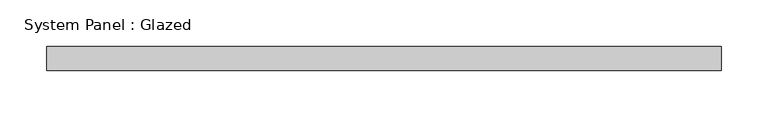
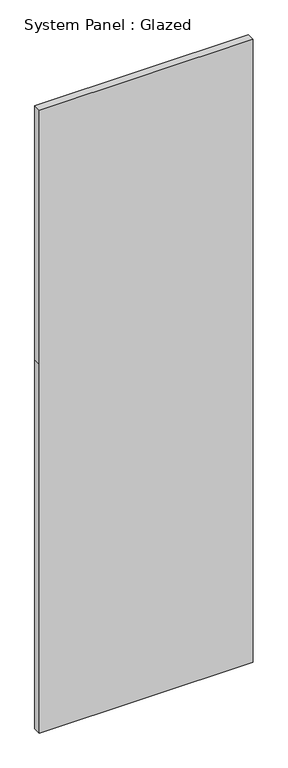
"""IFC4 building model written with IfcOpenShell, lengths in millimetres: plate geometry, System Panel : Glazed."""

from ifc_helpers import new_model, si_unit, frame, origin, place, context, project, spatial, polyline, outline, extrude, source, transform, mapped, element, save


def system_panel_glazed_9a0fbd8e(model_context):
    return source(origin(), model_context, "Body", "SweptSolid", [
        extrude(outline(polyline([(0.0, -358.775), (0.0, 358.775), (1308.1, 358.775), (2209.8, 358.775), (2209.8, -358.775), (1308.1, -358.775), (0.0, -358.775)])), frame((0.0, 19.05, 0.0), z_axis=(0.0, 1.0, 0.0), x_axis=(0.0, 0.0, 1.0)), (0.0, 0.0, 1.0), 25.4),
    ])


if __name__ == "__main__":
    model = new_model("IFC4")
    model_context = context("Model", 3, world=origin())
    ifc_project = project(units=[si_unit("LENGTHUNIT", "METRE", prefix="MILLI")], contexts=[model_context])
    site = spatial("IfcSite", under=ifc_project)
    building = spatial("IfcBuilding", under=site)
    placement = place(None, origin())
    system_panel_glazed_shape = system_panel_glazed_9a0fbd8e(model_context)
    element("IfcPlate", 1, ObjectType="System Panel : Glazed", at=placement, inside=building, context=model_context, shape_type="MappedRepresentation", body=[
        mapped(system_panel_glazed_shape, transform((0.0, 0.0, 0.0), x_axis=(1.0, 0.0, 0.0), y_axis=(0.0, 1.0, 0.0), z_axis=(0.0, 0.0, 1.0))),
    ])
    save(model, "model.ifc")

# Revit data of these elements
# Type "System Panel : Glazed"
#   Construction Type Id = "GSP4R"
#   Analytic Construction = "1/8 in Pilkington single glazing"
#   Visual Light Transmittance = 0.9
#   Solar Heat Gain Coefficient = 0.86
#   Heat Transfer Coefficient (U) = 1.18115 BTU/(h·ft²·°F)
#   Define Thermal Properties by = 1
# Element 1 (IfcPlate, "System Panel : Glazed")
#   Materials on its faces: "Glass"
# Materials
#   "Glass": class "Glass", colour RGB 0 128 192, transparency 0.75, Description = "Soda Lime Glass", Cost = 0
